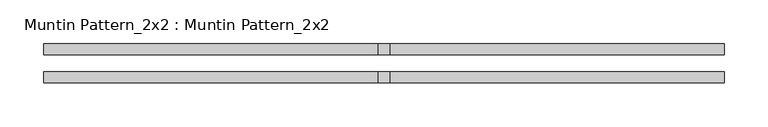
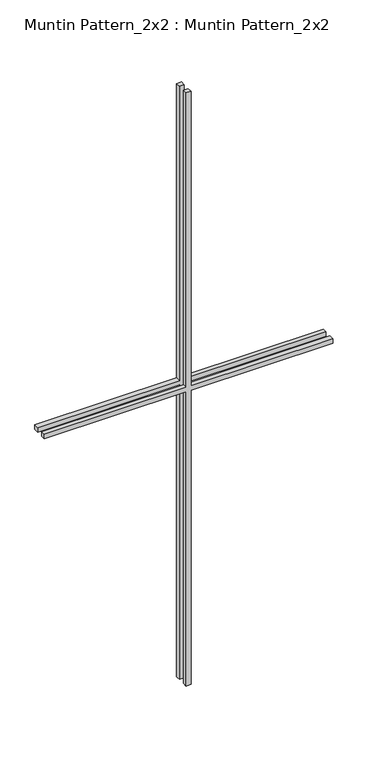
"""IFC4 building model written with IfcOpenShell, lengths in millimetres: proxy geometry, Muntin Pattern_2x2 : Muntin Pattern_2x2."""

from ifc_helpers import new_model, si_unit, frame, origin, place, context, project, spatial, polyline, outline, extrude, source, transform, mapped, element, save


def muntin_pattern_2x2_muntin_pattern_2x2_0a037076(model_context):
    return source(origin(), model_context, "Body", "SweptSolid", [
        extrude(outline(polyline([(850.9, -6.35), (850.9, -388.9375), (838.2, -388.9375), (838.2, -6.35), (0.0, -6.35), (0.0, 6.35), (838.2, 6.35), (838.2, 388.9375), (850.9, 388.9375), (850.9, 6.35), (1689.1, 6.35), (1689.1, -6.35), (850.9, -6.35)])), frame((0.0, 9.525, 0.0), z_axis=(0.0, 1.0, 0.0), x_axis=(0.0, 0.0, 1.0)), (0.0, 0.0, 1.0), 12.7),
        extrude(outline(polyline([(850.9, -6.35), (850.9, -388.9375), (838.2, -388.9375), (838.2, -6.35), (0.0, -6.35), (0.0, 6.35), (838.2, 6.35), (838.2, 388.9375), (850.9, 388.9375), (850.9, 6.35), (1689.1, 6.35), (1689.1, -6.35), (850.9, -6.35)])), frame((0.0, -22.225, 0.0), z_axis=(0.0, 1.0, 0.0), x_axis=(0.0, 0.0, 1.0)), (0.0, 0.0, 1.0), 12.7),
    ])


if __name__ == "__main__":
    model = new_model("IFC4")
    model_context = context("Model", 3, world=origin())
    ifc_project = project(units=[si_unit("LENGTHUNIT", "METRE", prefix="MILLI")], contexts=[model_context])
    site = spatial("IfcSite", under=ifc_project)
    building = spatial("IfcBuilding", under=site)
    placement = place(None, origin())
    muntin_pattern_2x2_muntin_pattern_2x2_shape = muntin_pattern_2x2_muntin_pattern_2x2_0a037076(model_context)
    element("IfcBuildingElementProxy", 1, Name="Muntin Pattern_2x2 : Muntin Pattern_2x2", ObjectType="Muntin Pattern_2x2 : Muntin Pattern_2x2", at=placement, inside=building, context=model_context, shape_type="MappedRepresentation", body=[
        mapped(muntin_pattern_2x2_muntin_pattern_2x2_shape, transform((0.0, 0.0, 0.0), x_axis=(1.0, 0.0, 0.0), y_axis=(0.0, 1.0, 0.0), z_axis=(0.0, 0.0, 1.0))),
    ])
    save(model, "model.ifc")

# Revit data of these elements
# Type "Muntin Pattern_2x2 : Muntin Pattern_2x2"
#   Width [instance default] = 4' - 0"
#   Thickness = 0' - 0 1/2"
#   Height [instance default] = 4' - 0"
#   Distance = 0' - 0 3/4"
#   Interior Material [instance default] = none
#   Exterior Material [instance default] = none
#   Default Elevation = 0
# Element 1 (IfcBuildingElementProxy, "Muntin Pattern_2x2 : Muntin Pattern_2x2")
#   Width = 2' - 6 5/8"
#   Height = 5' - 6 1/2"
#   Interior Material = Wood - Stained
#   Exterior Material = Clad - White
#   Materials on its faces: "Clad - White", "Wood - Stained"
# Materials
#   "Clad - White": class "Wood", colour RGB 242 242 238, transparency 0, Cost = 0
#   "Wood - Stained": class "Wood", colour RGB 224 178 126, transparency 0, Cost = 0
